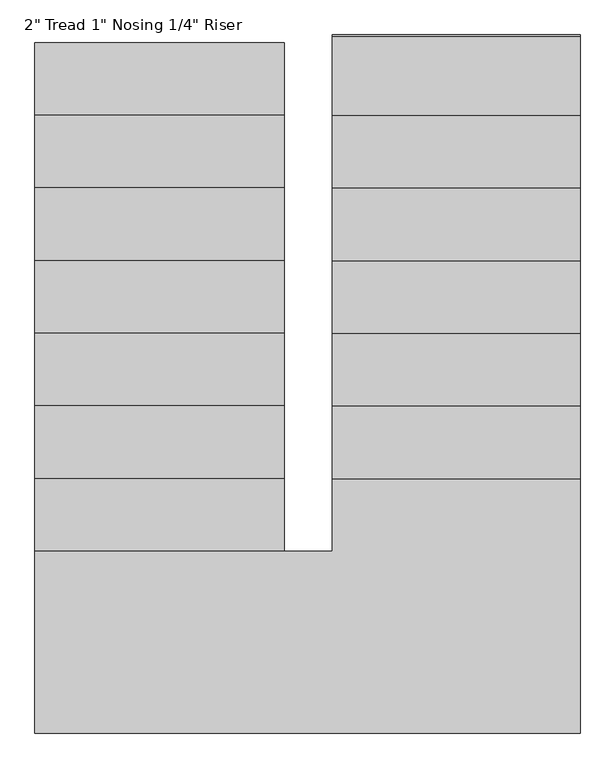
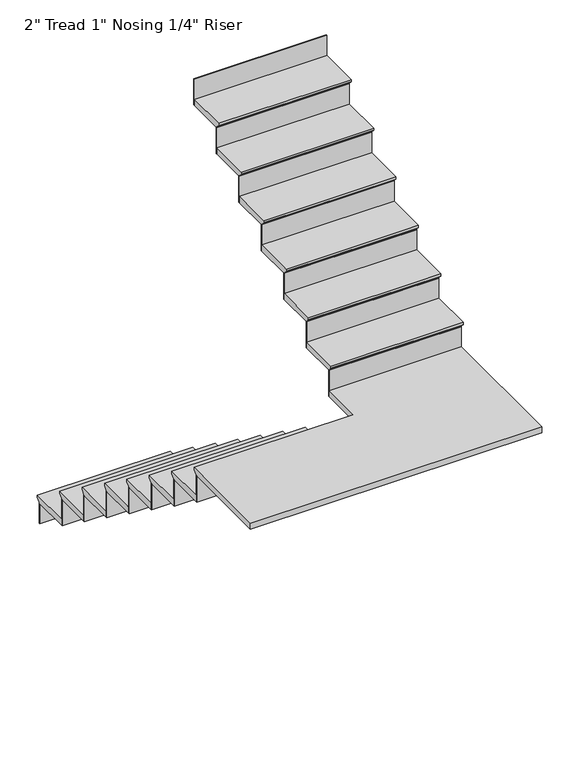
"""IFC4 building model written with IfcOpenShell, lengths in millimetres: stair flight geometry."""

from ifc_helpers import new_model, si_unit, origin, place, context, project, spatial, faceted_brep, source, transform, mapped, element, save


def stair_flight_d468406d(model_context):
    return source(origin(), model_context, "Body", "Brep", [
        faceted_brep([(-4232.280864, -3571.6080018, 198.6642857), (-4232.280864, -3571.6080018, 217.7142857), (-3187.6083919, -3571.6080018, 217.7142857), (-3187.6083919, -3571.6080018, 198.6642857), (-4232.280864, -3597.0080018, 173.2642857), (-3187.6083919, -3597.0080018, 173.2642857), (-4232.280864, -3901.8080018, 217.7142857), (-3187.6083919, -3901.8080018, 217.7142857), (-3187.6083919, -3597.0080018, 166.9142857), (-3187.6083919, -3901.8080018, 166.9142857), (-4232.280864, -3901.8080018, 166.9142857), (-4232.280864, -3597.0080018, 166.9142857)], [[[0, 1, 2, 3]], [[4, 0, 3, 5]], [[2, 1, 6, 7]], [[8, 9, 10, 11]], [[2, 7, 9, 8, 5, 3]], [[8, 11, 4, 5]], [[6, 1, 0, 4, 11, 10]], [[7, 6, 10, 9]]]),
        faceted_brep([(-4232.280864, -3597.0080018, 166.9142857), (-4232.280864, -3597.0080018, 0.0), (-4232.280864, -3603.3580018, 0.0), (-4232.280864, -3603.3580018, 166.9142857), (-3187.6083919, -3597.0080018, 166.9142857), (-3187.6083919, -3603.3580018, 166.9142857), (-3187.6083919, -3603.3580018, 0.0), (-3187.6083919, -3597.0080018, 0.0)], [[[0, 1, 2, 3]], [[4, 5, 6, 7]], [[1, 0, 4, 7]], [[2, 1, 7, 6]], [[3, 2, 6, 5]], [[0, 3, 5, 4]]]),
        faceted_brep([(-4232.280864, -3901.8080018, 384.6285714), (-4232.280864, -3901.8080018, 166.9142857), (-4232.280864, -3908.1580018, 166.9142857), (-4232.280864, -3908.1580018, 384.6285714), (-3187.6083919, -3901.8080018, 384.6285714), (-3187.6083919, -3908.1580018, 384.6285714), (-3187.6083919, -3908.1580018, 166.9142857), (-3187.6083919, -3901.8080018, 166.9142857)], [[[0, 1, 2, 3]], [[4, 5, 6, 7]], [[1, 0, 4, 7]], [[2, 1, 7, 6]], [[3, 2, 6, 5]], [[0, 3, 5, 4]]]),
        faceted_brep([(-3187.6083919, -3876.4080018, 435.4285714), (-4232.280864, -3876.4080018, 435.4285714), (-4232.280864, -4206.6080018, 435.4285714), (-3187.6083919, -4206.6080018, 435.4285714), (-3187.6083919, -3901.8080018, 384.6285714), (-3187.6083919, -4206.6080018, 384.6285714), (-4232.280864, -4206.6080018, 384.6285714), (-4232.280864, -3901.8080018, 384.6285714), (-3187.6083919, -3901.8080018, 390.9785714), (-3187.6083919, -3876.4080018, 416.3785714), (-4232.280864, -3901.8080018, 390.9785714), (-4232.280864, -3876.4080018, 416.3785714)], [[[0, 1, 2, 3]], [[4, 5, 6, 7]], [[0, 3, 5, 4, 8, 9]], [[4, 7, 10, 8]], [[2, 1, 11, 10, 7, 6]], [[3, 2, 6, 5]], [[11, 1, 0, 9]], [[10, 11, 9, 8]]]),
        faceted_brep([(-4232.280864, -4206.6080018, 602.3428571), (-4232.280864, -4206.6080018, 384.6285714), (-4232.280864, -4212.9580018, 384.6285714), (-4232.280864, -4212.9580018, 602.3428571), (-3187.6083919, -4206.6080018, 602.3428571), (-3187.6083919, -4212.9580018, 602.3428571), (-3187.6083919, -4212.9580018, 384.6285714), (-3187.6083919, -4206.6080018, 384.6285714)], [[[0, 1, 2, 3]], [[4, 5, 6, 7]], [[1, 0, 4, 7]], [[2, 1, 7, 6]], [[3, 2, 6, 5]], [[0, 3, 5, 4]]]),
        faceted_brep([(-3187.6083919, -4181.2080018, 653.1428571), (-4232.280864, -4181.2080018, 653.1428571), (-4232.280864, -4511.4080018, 653.1428571), (-3187.6083919, -4511.4080018, 653.1428571), (-3187.6083919, -4206.6080018, 602.3428571), (-3187.6083919, -4511.4080018, 602.3428571), (-4232.280864, -4511.4080018, 602.3428571), (-4232.280864, -4206.6080018, 602.3428571), (-3187.6083919, -4206.6080018, 608.6928571), (-3187.6083919, -4181.2080018, 634.0928571), (-4232.280864, -4206.6080018, 608.6928571), (-4232.280864, -4181.2080018, 634.0928571)], [[[0, 1, 2, 3]], [[4, 5, 6, 7]], [[0, 3, 5, 4, 8, 9]], [[4, 7, 10, 8]], [[2, 1, 11, 10, 7, 6]], [[3, 2, 6, 5]], [[11, 1, 0, 9]], [[10, 11, 9, 8]]]),
        faceted_brep([(-4232.280864, -4511.4080018, 820.0571429), (-4232.280864, -4511.4080018, 602.3428571), (-4232.280864, -4517.7580018, 602.3428571), (-4232.280864, -4517.7580018, 820.0571429), (-3187.6083919, -4511.4080018, 820.0571429), (-3187.6083919, -4517.7580018, 820.0571429), (-3187.6083919, -4517.7580018, 602.3428571), (-3187.6083919, -4511.4080018, 602.3428571)], [[[0, 1, 2, 3]], [[4, 5, 6, 7]], [[1, 0, 4, 7]], [[2, 1, 7, 6]], [[3, 2, 6, 5]], [[0, 3, 5, 4]]]),
        faceted_brep([(-3187.6083919, -4486.0080018, 870.8571429), (-4232.280864, -4486.0080018, 870.8571429), (-4232.280864, -4816.2080018, 870.8571429), (-3187.6083919, -4816.2080018, 870.8571429), (-3187.6083919, -4511.4080018, 820.0571429), (-3187.6083919, -4816.2080018, 820.0571429), (-4232.280864, -4816.2080018, 820.0571429), (-4232.280864, -4511.4080018, 820.0571429), (-3187.6083919, -4511.4080018, 826.4071429), (-3187.6083919, -4486.0080018, 851.8071429), (-4232.280864, -4511.4080018, 826.4071429), (-4232.280864, -4486.0080018, 851.8071429)], [[[0, 1, 2, 3]], [[4, 5, 6, 7]], [[0, 3, 5, 4, 8, 9]], [[4, 7, 10, 8]], [[2, 1, 11, 10, 7, 6]], [[3, 2, 6, 5]], [[11, 1, 0, 9]], [[10, 11, 9, 8]]]),
        faceted_brep([(-4232.280864, -4816.2080018, 1037.7714286), (-4232.280864, -4816.2080018, 820.0571429), (-4232.280864, -4822.5580018, 820.0571429), (-4232.280864, -4822.5580018, 1037.7714286), (-3187.6083919, -4816.2080018, 1037.7714286), (-3187.6083919, -4822.5580018, 1037.7714286), (-3187.6083919, -4822.5580018, 820.0571429), (-3187.6083919, -4816.2080018, 820.0571429)], [[[0, 1, 2, 3]], [[4, 5, 6, 7]], [[1, 0, 4, 7]], [[2, 1, 7, 6]], [[3, 2, 6, 5]], [[0, 3, 5, 4]]]),
        faceted_brep([(-3187.6083919, -4790.8080018, 1088.5714286), (-4232.280864, -4790.8080018, 1088.5714286), (-4232.280864, -5121.0080018, 1088.5714286), (-3187.6083919, -5121.0080018, 1088.5714286), (-3187.6083919, -4816.2080018, 1037.7714286), (-3187.6083919, -5121.0080018, 1037.7714286), (-4232.280864, -5121.0080018, 1037.7714286), (-4232.280864, -4816.2080018, 1037.7714286), (-3187.6083919, -4816.2080018, 1044.1214286), (-3187.6083919, -4790.8080018, 1069.5214286), (-4232.280864, -4816.2080018, 1044.1214286), (-4232.280864, -4790.8080018, 1069.5214286)], [[[0, 1, 2, 3]], [[4, 5, 6, 7]], [[0, 3, 5, 4, 8, 9]], [[4, 7, 10, 8]], [[2, 1, 11, 10, 7, 6]], [[3, 2, 6, 5]], [[11, 1, 0, 9]], [[10, 11, 9, 8]]]),
        faceted_brep([(-4232.280864, -5121.0080018, 1255.4857143), (-4232.280864, -5121.0080018, 1037.7714286), (-4232.280864, -5127.3580018, 1037.7714286), (-4232.280864, -5127.3580018, 1255.4857143), (-3187.6083919, -5121.0080018, 1255.4857143), (-3187.6083919, -5127.3580018, 1255.4857143), (-3187.6083919, -5127.3580018, 1037.7714286), (-3187.6083919, -5121.0080018, 1037.7714286)], [[[0, 1, 2, 3]], [[4, 5, 6, 7]], [[1, 0, 4, 7]], [[2, 1, 7, 6]], [[3, 2, 6, 5]], [[0, 3, 5, 4]]]),
        faceted_brep([(-3187.6083919, -5095.6080018, 1306.2857143), (-4232.280864, -5095.6080018, 1306.2857143), (-4232.280864, -5425.8080018, 1306.2857143), (-3187.6083919, -5425.8080018, 1306.2857143), (-3187.6083919, -5121.0080018, 1255.4857143), (-3187.6083919, -5425.8080018, 1255.4857143), (-4232.280864, -5425.8080018, 1255.4857143), (-4232.280864, -5121.0080018, 1255.4857143), (-3187.6083919, -5121.0080018, 1261.8357143), (-3187.6083919, -5095.6080018, 1287.2357143), (-4232.280864, -5121.0080018, 1261.8357143), (-4232.280864, -5095.6080018, 1287.2357143)], [[[0, 1, 2, 3]], [[4, 5, 6, 7]], [[0, 3, 5, 4, 8, 9]], [[4, 7, 10, 8]], [[2, 1, 11, 10, 7, 6]], [[3, 2, 6, 5]], [[11, 1, 0, 9]], [[10, 11, 9, 8]]]),
        faceted_brep([(-4232.280864, -5425.8080018, 1473.2), (-4232.280864, -5425.8080018, 1255.4857143), (-4232.280864, -5432.1580018, 1255.4857143), (-4232.280864, -5432.1580018, 1473.2), (-3187.6083919, -5425.8080018, 1473.2), (-3187.6083919, -5432.1580018, 1473.2), (-3187.6083919, -5432.1580018, 1255.4857143), (-3187.6083919, -5425.8080018, 1255.4857143)], [[[0, 1, 2, 3]], [[4, 5, 6, 7]], [[1, 0, 4, 7]], [[2, 1, 7, 6]], [[3, 2, 6, 5]], [[0, 3, 5, 4]]]),
        faceted_brep([(-3187.6083919, -5400.4080018, 1524.0), (-4232.280864, -5400.4080018, 1524.0), (-4232.280864, -5730.6080018, 1524.0), (-3187.6083919, -5730.6080018, 1524.0), (-3187.6083919, -5425.8080018, 1473.2), (-3187.6083919, -5730.6080018, 1473.2), (-4232.280864, -5730.6080018, 1473.2), (-4232.280864, -5425.8080018, 1473.2), (-3187.6083919, -5425.8080018, 1479.55), (-3187.6083919, -5400.4080018, 1504.95), (-4232.280864, -5425.8080018, 1479.55), (-4232.280864, -5400.4080018, 1504.95)], [[[0, 1, 2, 3]], [[4, 5, 6, 7]], [[0, 3, 5, 4, 8, 9]], [[4, 7, 10, 8]], [[2, 1, 11, 10, 7, 6]], [[3, 2, 6, 5]], [[11, 1, 0, 9]], [[10, 11, 9, 8]]]),
        faceted_brep([(-4232.280864, -5730.6080018, 1690.9142857), (-4232.280864, -5730.6080018, 1473.2), (-4232.280864, -5736.9580018, 1473.2), (-4232.280864, -5736.9580018, 1690.9142857), (-3187.6083919, -5730.6080018, 1690.9142857), (-3187.6083919, -5736.9580018, 1690.9142857), (-3187.6083919, -5736.9580018, 1473.2), (-3187.6083919, -5730.6080018, 1473.2)], [[[0, 1, 2, 3]], [[4, 5, 6, 7]], [[1, 0, 4, 7]], [[2, 1, 7, 6]], [[3, 2, 6, 5]], [[0, 3, 5, 4]]]),
        faceted_brep([(-2984.4083919, -5375.0080018, 1741.7142857), (-2984.4083919, -5705.2080018, 1741.7142857), (-4232.280864, -5705.2080018, 1741.7142857), (-4232.280864, -6467.2080018, 1741.7142857), (-1946.280864, -6467.2080018, 1741.7142857), (-1946.280864, -5375.0080018, 1741.7142857), (-2984.4083919, -5705.2080018, 1690.9142857), (-2984.4083919, -5375.0080018, 1690.9142857), (-1946.280864, -5375.0080018, 1690.9142857), (-1946.280864, -6467.2080018, 1690.9142857), (-4232.280864, -6467.2080018, 1690.9142857), (-4232.280864, -5730.6080018, 1690.9142857), (-3187.6083919, -5730.6080018, 1690.9142857), (-3187.6083919, -5705.2080018, 1690.9142857), (-3187.6083919, -5705.2080018, 1722.6642857), (-4232.280864, -5705.2080018, 1722.6642857), (-3187.6083919, -5730.6080018, 1697.2642857), (-4232.280864, -5730.6080018, 1697.2642857)], [[[0, 1, 2, 3, 4, 5]], [[6, 7, 8, 9, 10, 11, 12, 13]], [[1, 0, 7, 6]], [[2, 1, 6, 13, 14, 15]], [[13, 12, 16, 14]], [[12, 11, 17, 16]], [[3, 2, 15, 17, 11, 10]], [[4, 3, 10, 9]], [[5, 4, 9, 8]], [[0, 5, 8, 7]], [[17, 15, 14, 16]]]),
        faceted_brep([(-1946.280864, -5375.0080018, 1908.6285714), (-1946.280864, -5375.0080018, 1690.9142857), (-1946.280864, -5368.6580018, 1690.9142857), (-1946.280864, -5368.6580018, 1908.6285714), (-2984.4083919, -5375.0080018, 1908.6285714), (-2984.4083919, -5368.6580018, 1908.6285714), (-2984.4083919, -5368.6580018, 1690.9142857), (-2984.4083919, -5375.0080018, 1690.9142857)], [[[0, 1, 2, 3]], [[4, 5, 6, 7]], [[1, 0, 4, 7]], [[2, 1, 7, 6]], [[3, 2, 6, 5]], [[0, 3, 5, 4]]]),
        faceted_brep([(-2984.4083919, -5400.4080018, 1959.4285714), (-1946.280864, -5400.4080018, 1959.4285714), (-1946.280864, -5070.2080018, 1959.4285714), (-2984.4083919, -5070.2080018, 1959.4285714), (-2984.4083919, -5375.0080018, 1908.6285714), (-2984.4083919, -5070.2080018, 1908.6285714), (-1946.280864, -5070.2080018, 1908.6285714), (-1946.280864, -5375.0080018, 1908.6285714), (-2984.4083919, -5375.0080018, 1914.9785714), (-2984.4083919, -5400.4080018, 1940.3785714), (-1946.280864, -5375.0080018, 1914.9785714), (-1946.280864, -5400.4080018, 1940.3785714)], [[[0, 1, 2, 3]], [[4, 5, 6, 7]], [[0, 3, 5, 4, 8, 9]], [[4, 7, 10, 8]], [[2, 1, 11, 10, 7, 6]], [[3, 2, 6, 5]], [[11, 1, 0, 9]], [[10, 11, 9, 8]]]),
        faceted_brep([(-1946.280864, -5070.2080018, 2126.3428571), (-1946.280864, -5070.2080018, 1908.6285714), (-1946.280864, -5063.8580018, 1908.6285714), (-1946.280864, -5063.8580018, 2126.3428571), (-2984.4083919, -5070.2080018, 2126.3428571), (-2984.4083919, -5063.8580018, 2126.3428571), (-2984.4083919, -5063.8580018, 1908.6285714), (-2984.4083919, -5070.2080018, 1908.6285714)], [[[0, 1, 2, 3]], [[4, 5, 6, 7]], [[1, 0, 4, 7]], [[2, 1, 7, 6]], [[3, 2, 6, 5]], [[0, 3, 5, 4]]]),
        faceted_brep([(-2984.4083919, -5095.6080018, 2177.1428571), (-1946.280864, -5095.6080018, 2177.1428571), (-1946.280864, -4765.4080018, 2177.1428571), (-2984.4083919, -4765.4080018, 2177.1428571), (-2984.4083919, -5070.2080018, 2126.3428571), (-2984.4083919, -4765.4080018, 2126.3428571), (-1946.280864, -4765.4080018, 2126.3428571), (-1946.280864, -5070.2080018, 2126.3428571), (-2984.4083919, -5070.2080018, 2132.6928571), (-2984.4083919, -5095.6080018, 2158.0928571), (-1946.280864, -5070.2080018, 2132.6928571), (-1946.280864, -5095.6080018, 2158.0928571)], [[[0, 1, 2, 3]], [[4, 5, 6, 7]], [[0, 3, 5, 4, 8, 9]], [[4, 7, 10, 8]], [[2, 1, 11, 10, 7, 6]], [[3, 2, 6, 5]], [[11, 1, 0, 9]], [[10, 11, 9, 8]]]),
        faceted_brep([(-1946.280864, -4765.4080018, 2344.0571429), (-1946.280864, -4765.4080018, 2126.3428571), (-1946.280864, -4759.0580018, 2126.3428571), (-1946.280864, -4759.0580018, 2344.0571429), (-2984.4083919, -4765.4080018, 2344.0571429), (-2984.4083919, -4759.0580018, 2344.0571429), (-2984.4083919, -4759.0580018, 2126.3428571), (-2984.4083919, -4765.4080018, 2126.3428571)], [[[0, 1, 2, 3]], [[4, 5, 6, 7]], [[1, 0, 4, 7]], [[2, 1, 7, 6]], [[3, 2, 6, 5]], [[0, 3, 5, 4]]]),
        faceted_brep([(-2984.4083919, -4790.8080018, 2394.8571429), (-1946.280864, -4790.8080018, 2394.8571429), (-1946.280864, -4460.6080018, 2394.8571429), (-2984.4083919, -4460.6080018, 2394.8571429), (-2984.4083919, -4765.4080018, 2344.0571429), (-2984.4083919, -4460.6080018, 2344.0571429), (-1946.280864, -4460.6080018, 2344.0571429), (-1946.280864, -4765.4080018, 2344.0571429), (-2984.4083919, -4765.4080018, 2350.4071429), (-2984.4083919, -4790.8080018, 2375.8071429), (-1946.280864, -4765.4080018, 2350.4071429), (-1946.280864, -4790.8080018, 2375.8071429)], [[[0, 1, 2, 3]], [[4, 5, 6, 7]], [[0, 3, 5, 4, 8, 9]], [[4, 7, 10, 8]], [[2, 1, 11, 10, 7, 6]], [[3, 2, 6, 5]], [[11, 1, 0, 9]], [[10, 11, 9, 8]]]),
        faceted_brep([(-1946.280864, -4460.6080018, 2561.7714286), (-1946.280864, -4460.6080018, 2344.0571429), (-1946.280864, -4454.2580018, 2344.0571429), (-1946.280864, -4454.2580018, 2561.7714286), (-2984.4083919, -4460.6080018, 2561.7714286), (-2984.4083919, -4454.2580018, 2561.7714286), (-2984.4083919, -4454.2580018, 2344.0571429), (-2984.4083919, -4460.6080018, 2344.0571429)], [[[0, 1, 2, 3]], [[4, 5, 6, 7]], [[1, 0, 4, 7]], [[2, 1, 7, 6]], [[3, 2, 6, 5]], [[0, 3, 5, 4]]]),
        faceted_brep([(-2984.4083919, -4486.0080018, 2612.5714286), (-1946.280864, -4486.0080018, 2612.5714286), (-1946.280864, -4155.8080018, 2612.5714286), (-2984.4083919, -4155.8080018, 2612.5714286), (-2984.4083919, -4460.6080018, 2561.7714286), (-2984.4083919, -4155.8080018, 2561.7714286), (-1946.280864, -4155.8080018, 2561.7714286), (-1946.280864, -4460.6080018, 2561.7714286), (-2984.4083919, -4460.6080018, 2568.1214286), (-2984.4083919, -4486.0080018, 2593.5214286), (-1946.280864, -4460.6080018, 2568.1214286), (-1946.280864, -4486.0080018, 2593.5214286)], [[[0, 1, 2, 3]], [[4, 5, 6, 7]], [[0, 3, 5, 4, 8, 9]], [[4, 7, 10, 8]], [[2, 1, 11, 10, 7, 6]], [[3, 2, 6, 5]], [[11, 1, 0, 9]], [[10, 11, 9, 8]]]),
        faceted_brep([(-1946.280864, -4155.8080018, 2779.4857143), (-1946.280864, -4155.8080018, 2561.7714286), (-1946.280864, -4149.4580018, 2561.7714286), (-1946.280864, -4149.4580018, 2779.4857143), (-2984.4083919, -4155.8080018, 2779.4857143), (-2984.4083919, -4149.4580018, 2779.4857143), (-2984.4083919, -4149.4580018, 2561.7714286), (-2984.4083919, -4155.8080018, 2561.7714286)], [[[0, 1, 2, 3]], [[4, 5, 6, 7]], [[1, 0, 4, 7]], [[2, 1, 7, 6]], [[3, 2, 6, 5]], [[0, 3, 5, 4]]]),
        faceted_brep([(-2984.4083919, -4181.2080018, 2830.2857143), (-1946.280864, -4181.2080018, 2830.2857143), (-1946.280864, -3851.0080018, 2830.2857143), (-2984.4083919, -3851.0080018, 2830.2857143), (-2984.4083919, -4155.8080018, 2779.4857143), (-2984.4083919, -3851.0080018, 2779.4857143), (-1946.280864, -3851.0080018, 2779.4857143), (-1946.280864, -4155.8080018, 2779.4857143), (-2984.4083919, -4155.8080018, 2785.8357143), (-2984.4083919, -4181.2080018, 2811.2357143), (-1946.280864, -4155.8080018, 2785.8357143), (-1946.280864, -4181.2080018, 2811.2357143)], [[[0, 1, 2, 3]], [[4, 5, 6, 7]], [[0, 3, 5, 4, 8, 9]], [[4, 7, 10, 8]], [[2, 1, 11, 10, 7, 6]], [[3, 2, 6, 5]], [[11, 1, 0, 9]], [[10, 11, 9, 8]]]),
        faceted_brep([(-1946.280864, -3851.0080018, 2997.2), (-1946.280864, -3851.0080018, 2779.4857143), (-1946.280864, -3844.6580018, 2779.4857143), (-1946.280864, -3844.6580018, 2997.2), (-2984.4083919, -3851.0080018, 2997.2), (-2984.4083919, -3844.6580018, 2997.2), (-2984.4083919, -3844.6580018, 2779.4857143), (-2984.4083919, -3851.0080018, 2779.4857143)], [[[0, 1, 2, 3]], [[4, 5, 6, 7]], [[1, 0, 4, 7]], [[2, 1, 7, 6]], [[3, 2, 6, 5]], [[0, 3, 5, 4]]]),
        faceted_brep([(-1946.280864, -3546.2080018, 3214.9142857), (-1946.280864, -3546.2080018, 2997.2), (-1946.280864, -3539.8580018, 2997.2), (-1946.280864, -3539.8580018, 3214.9142857), (-2984.4083919, -3546.2080018, 3214.9142857), (-2984.4083919, -3539.8580018, 3214.9142857), (-2984.4083919, -3539.8580018, 2997.2), (-2984.4083919, -3546.2080018, 2997.2)], [[[0, 1, 2, 3]], [[4, 5, 6, 7]], [[1, 0, 4, 7]], [[2, 1, 7, 6]], [[3, 2, 6, 5]], [[0, 3, 5, 4]]]),
        faceted_brep([(-2984.4083919, -3876.4080018, 3048.0), (-1946.280864, -3876.4080018, 3048.0), (-1946.280864, -3546.2080018, 3048.0), (-2984.4083919, -3546.2080018, 3048.0), (-2984.4083919, -3851.0080018, 2997.2), (-2984.4083919, -3546.2080018, 2997.2), (-1946.280864, -3546.2080018, 2997.2), (-1946.280864, -3851.0080018, 2997.2), (-2984.4083919, -3851.0080018, 3003.55), (-2984.4083919, -3876.4080018, 3028.95), (-1946.280864, -3851.0080018, 3003.55), (-1946.280864, -3876.4080018, 3028.95)], [[[0, 1, 2, 3]], [[4, 5, 6, 7]], [[0, 3, 5, 4, 8, 9]], [[4, 7, 10, 8]], [[2, 1, 11, 10, 7, 6]], [[3, 2, 6, 5]], [[11, 1, 0, 9]], [[10, 11, 9, 8]]]),
    ])


if __name__ == "__main__":
    model = new_model("IFC4")
    model_context = context("Model", 3, world=origin())
    ifc_project = project(units=[si_unit("LENGTHUNIT", "METRE", prefix="MILLI")], contexts=[model_context])
    site = spatial("IfcSite", under=ifc_project)
    building = spatial("IfcBuilding", under=site)
    placement = place(None, origin())
    stair_flight_shape = stair_flight_d468406d(model_context)
    element("IfcStairFlight", 1, ObjectType="2\" Tread 1\" Nosing 1/4\" Riser", at=placement, inside=building, context=model_context, shape_type="MappedRepresentation", body=[
        mapped(stair_flight_shape, transform((0.0, 0.0, 0.0), x_axis=(1.0, 0.0, 0.0), y_axis=(0.0, 1.0, 0.0), z_axis=(0.0, 0.0, 1.0))),
    ])
    save(model, "model.ifc")
